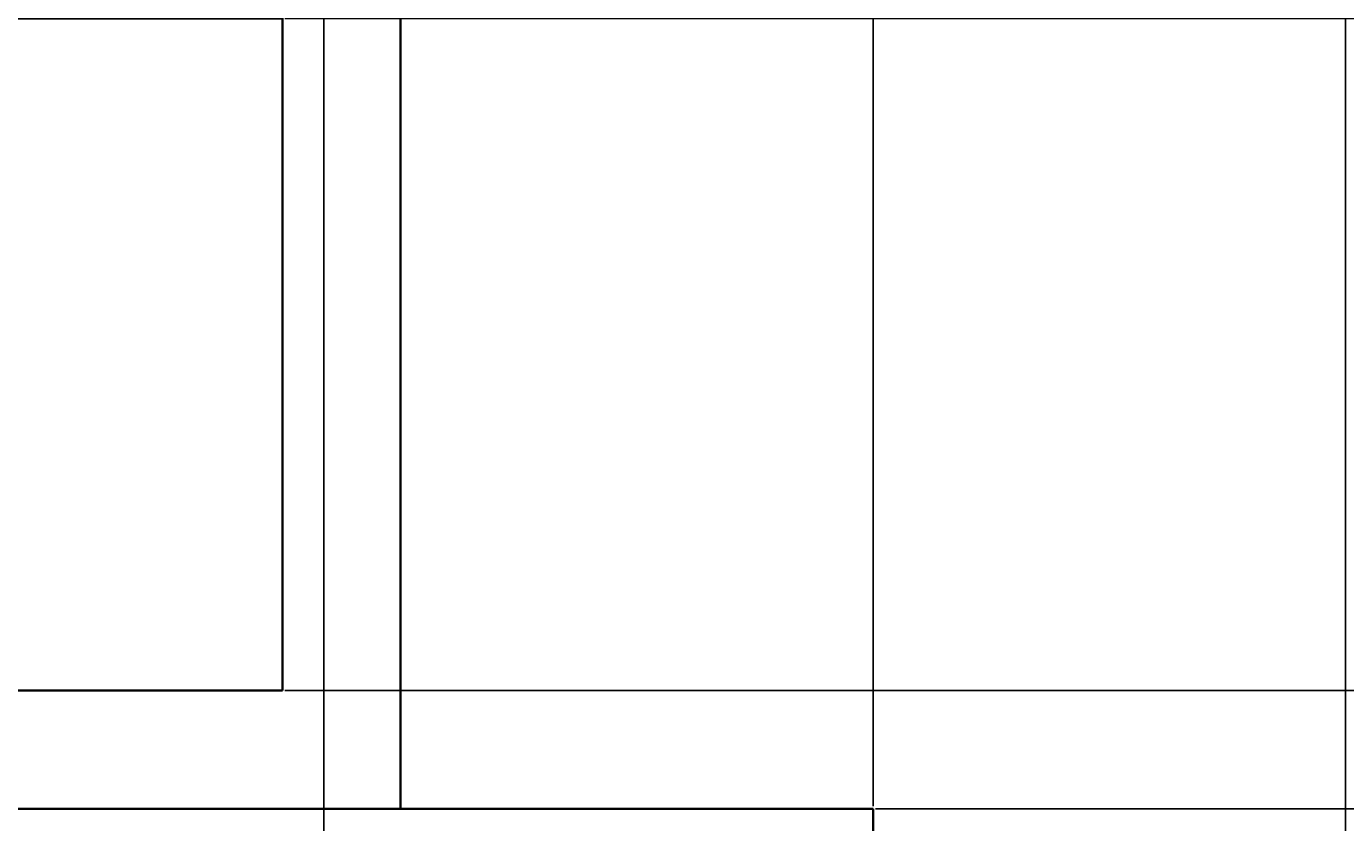
# Model space of a CAD drawing. Units: inches. Extents: x -6 to 289, y -8 to 323.
# Tile 65 of 107: x 238 to 271, y 139 to 159. Entities that reach past the tile are written whole.
import ezdxf

# ---------------------------------------------------------------- set-up
doc = ezdxf.new("R2010")
doc.units = ezdxf.units.IN
doc.header["$MEASUREMENT"] = 0
doc.layers.add('A-ANNO-DIMS', color=2, linetype='Continuous', lineweight=18)
doc.layers.add('A-ELEV', color=7, linetype='Continuous', lineweight=35)
doc.styles.get("Standard").update_dxf_attribs({"font": 'arial.ttf'})
doc.dimstyles.get("Standard").update_dxf_attribs({"dimtxt": 0.18, "dimasz": 0.18, "dimexe": 0.18, "dimexo": 0.0625, "dimgap": 0.09, "dimtad": 0, "dimtih": 1, "dimtoh": 1, "dimdec": 4, "dimzin": 0, "dimdsep": 46, "dimtxsty": 'Standard', "dimcen": 0.09, "dimadec": 0, "dimazin": 0, "dimtfac": 1, "dimtdec": 4, "dimtofl": 0, "dimtmove": 0, "dimatfit": 3, "dimfxl": 1, "dimtolj": 1, "dimtzin": 0, "dimarcsym": 0})

# ---------------------------------------------------------------- blocks, each defined once
blk = doc.blocks.new('*D15')
at = {"layer": 'A-ANNO-DIMS', "color": 0, "lineweight": -2, "transparency": 16777216}
for p, q in [((247.164, 162.411), (247.164, 322.969)), ((247.344, 322.789), (258.944, 322.789)), ((270.984, 322.789), (259.384, 322.789)), ((271.164, 7.351), (271.164, 322.969))]:
    blk.add_line(p, q, dxfattribs=at)
at = {"layer": 'A-ANNO-DIMS', "color": 0, "transparency": 16777216}
for points in [[(247.344, 322.819), (247.344, 322.759), (247.164, 322.789)], [(270.984, 322.819), (270.984, 322.759), (271.164, 322.789)]]:
    blk.add_solid(points, dxfattribs=at)
at = {"layer": 'Defpoints', "color": 0, "transparency": 16777216}
for p in [(271.164, 322.789), (247.164, 162.348), (271.164, 7.289)]:
    blk.add_point(p, dxfattribs=at)
at = {"layer": 'A-ANNO-DIMS', "color": 0, "transparency": 16777216, "insert": (259.164, 322.789), "char_height": 0.18, "attachment_point": 5}
blk.add_mtext('\\A1;24', dxfattribs=at)
blk = doc.blocks.new('*D24')
at = {"layer": 'A-ANNO-DIMS', "color": 0, "lineweight": -2, "transparency": 16777216}
for p, q in [((126.946, 178.654), (288.653, 178.654)), ((288.473, 178.474), (288.473, 159.153)), ((288.473, 139.469), (288.473, 158.789)), ((259.226, 139.289), (288.653, 139.289))]:
    blk.add_line(p, q, dxfattribs=at)
at = {"layer": 'A-ANNO-DIMS', "color": 0, "transparency": 16777216}
for points in [[(288.443, 178.474), (288.503, 178.474), (288.473, 178.654)], [(288.443, 139.469), (288.503, 139.469), (288.473, 139.289)]]:
    blk.add_solid(points, dxfattribs=at)
at = {"layer": 'Defpoints', "color": 0, "transparency": 16777216}
for p in [(126.883, 178.654), (288.473, 178.654), (259.164, 139.289)]:
    blk.add_point(p, dxfattribs=at)
at = {"layer": 'A-ANNO-DIMS', "color": 0, "transparency": 16777216, "insert": (288.473, 158.971), "char_height": 0.18, "attachment_point": 5}
blk.add_mtext('\\A1;39.365', dxfattribs=at)
blk = doc.blocks.new('*D81')
at = {"layer": 'A-ANNO-DIMS', "color": 0, "lineweight": -2, "transparency": 16777216}
for p, q in [((230.292, 68.842), (230.292, 322.969)), ((230.472, 322.789), (237.298, 322.789)), ((245.035, 322.789), (238.208, 322.789)), ((245.215, 66.286), (245.215, 322.969))]:
    blk.add_line(p, q, dxfattribs=at)
at = {"layer": 'A-ANNO-DIMS', "color": 0, "transparency": 16777216}
for points in [[(230.472, 322.819), (230.472, 322.759), (230.292, 322.789)], [(245.035, 322.819), (245.035, 322.759), (245.215, 322.789)]]:
    blk.add_solid(points, dxfattribs=at)
at = {"layer": 'Defpoints', "color": 0, "transparency": 16777216}
for p in [(245.215, 322.789), (230.292, 68.779), (245.215, 66.224)]:
    blk.add_point(p, dxfattribs=at)
at = {"layer": 'A-ANNO-DIMS', "color": 0, "transparency": 16777216, "insert": (237.753, 322.789), "char_height": 0.18, "attachment_point": 5}
blk.add_mtext('\\A1;14.923', dxfattribs=at)
blk = doc.blocks.new('*D82')
at = {"layer": 'A-ANNO-DIMS', "color": 0, "lineweight": -2, "transparency": 16777216}
for p, q in [((245.215, 66.286), (245.215, 322.969)), ((245.395, 322.789), (258.699, 322.789)), ((272.793, 322.789), (259.489, 322.789)), ((272.973, 66.286), (272.973, 322.969))]:
    blk.add_line(p, q, dxfattribs=at)
at = {"layer": 'A-ANNO-DIMS', "color": 0, "transparency": 16777216}
for points in [[(245.395, 322.819), (245.395, 322.759), (245.215, 322.789)], [(272.793, 322.819), (272.793, 322.759), (272.973, 322.789)]]:
    blk.add_solid(points, dxfattribs=at)
at = {"layer": 'Defpoints', "color": 0, "transparency": 16777216}
for p in [(272.973, 322.789), (245.215, 66.224), (272.973, 66.224)]:
    blk.add_point(p, dxfattribs=at)
at = {"layer": 'A-ANNO-DIMS', "color": 0, "transparency": 16777216, "insert": (259.094, 322.789), "char_height": 0.18, "attachment_point": 5}
blk.add_mtext('\\A1;27.76', dxfattribs=at)
blk = doc.blocks.new('*D100')
at = {"layer": 'A-ANNO-DIMS', "color": 0, "lineweight": -2, "transparency": 16777216}
for p, q in [((247.164, 162.411), (247.164, 322.969)), ((247.344, 322.789), (252.954, 322.789)), ((258.984, 322.789), (253.373, 322.789)), ((259.164, 139.351), (259.164, 322.969))]:
    blk.add_line(p, q, dxfattribs=at)
at = {"layer": 'A-ANNO-DIMS', "color": 0, "transparency": 16777216}
for points in [[(247.344, 322.819), (247.344, 322.759), (247.164, 322.789)], [(258.984, 322.819), (258.984, 322.759), (259.164, 322.789)]]:
    blk.add_solid(points, dxfattribs=at)
at = {"layer": 'Defpoints', "color": 0, "transparency": 16777216}
for p in [(259.164, 322.789), (247.164, 162.348), (259.164, 139.289)]:
    blk.add_point(p, dxfattribs=at)
at = {"layer": 'A-ANNO-DIMS', "color": 0, "transparency": 16777216, "insert": (253.164, 322.789), "char_height": 0.18, "attachment_point": 5}
blk.add_mtext('\\A1;12', dxfattribs=at)
blk = doc.blocks.new('*D101')
at = {"layer": 'A-ANNO-DIMS', "color": 0, "lineweight": -2, "transparency": 16777216}
for p, q in [((259.226, 139.289), (288.653, 139.289)), ((288.473, 139.109), (288.473, 133.469)), ((288.473, 127.469), (288.473, 133.108)), ((259.226, 127.289), (288.653, 127.289))]:
    blk.add_line(p, q, dxfattribs=at)
at = {"layer": 'A-ANNO-DIMS', "color": 0, "transparency": 16777216}
for points in [[(288.443, 139.109), (288.503, 139.109), (288.473, 139.289)], [(288.443, 127.469), (288.503, 127.469), (288.473, 127.289)]]:
    blk.add_solid(points, dxfattribs=at)
at = {"layer": 'Defpoints', "color": 0, "transparency": 16777216}
for p in [(259.164, 139.289), (288.473, 139.289), (259.164, 127.289)]:
    blk.add_point(p, dxfattribs=at)
at = {"layer": 'A-ANNO-DIMS', "color": 0, "transparency": 16777216, "insert": (288.473, 133.289), "char_height": 0.18, "attachment_point": 5}
blk.add_mtext('\\A1;12', dxfattribs=at)
blk = doc.blocks.new('*D102')
at = {"layer": 'A-ANNO-DIMS', "color": 0, "lineweight": -2, "transparency": 16777216}
for p, q in [((244.226, 142.289), (288.653, 142.289)), ((288.473, 142.109), (288.473, 140.971)), ((288.473, 139.469), (288.473, 140.607)), ((259.226, 139.289), (288.653, 139.289))]:
    blk.add_line(p, q, dxfattribs=at)
at = {"layer": 'A-ANNO-DIMS', "color": 0, "transparency": 16777216}
for points in [[(288.443, 142.109), (288.503, 142.109), (288.473, 142.289)], [(288.443, 139.469), (288.503, 139.469), (288.473, 139.289)]]:
    blk.add_solid(points, dxfattribs=at)
at = {"layer": 'Defpoints', "color": 0, "transparency": 16777216}
for p in [(244.164, 142.289), (288.473, 142.289), (259.164, 139.289)]:
    blk.add_point(p, dxfattribs=at)
at = {"layer": 'A-ANNO-DIMS', "color": 0, "transparency": 16777216, "insert": (288.473, 140.789), "char_height": 0.18, "attachment_point": 5}
blk.add_mtext('\\A1;3', dxfattribs=at)
blk = doc.blocks.new('*D103')
at = {"layer": 'A-ANNO-DIMS', "color": 0, "lineweight": -2, "transparency": 16777216}
for p, q in [((244.226, 159.348), (288.653, 159.348)), ((288.473, 159.168), (288.473, 151)), ((288.473, 142.469), (288.473, 150.637)), ((244.226, 142.289), (288.653, 142.289))]:
    blk.add_line(p, q, dxfattribs=at)
at = {"layer": 'A-ANNO-DIMS', "color": 0, "transparency": 16777216}
for points in [[(288.443, 159.168), (288.503, 159.168), (288.473, 159.348)], [(288.443, 142.469), (288.503, 142.469), (288.473, 142.289)]]:
    blk.add_solid(points, dxfattribs=at)
at = {"layer": 'Defpoints', "color": 0, "transparency": 16777216}
for p in [(244.164, 159.348), (288.473, 159.348), (244.164, 142.289)]:
    blk.add_point(p, dxfattribs=at)
at = {"layer": 'A-ANNO-DIMS', "color": 0, "transparency": 16777216, "insert": (288.473, 150.819), "char_height": 0.18, "attachment_point": 5}
blk.add_mtext('\\A1;17.06', dxfattribs=at)

msp = doc.modelspace()

# ---------------------------------------------------------------- linework, layer by layer
at = {"layer": 'A-ELEV'}
for p, q in [((247.1638, 139.2888), (247.1638, 247.2888)), ((115.1638, 139.2888), (259.1638, 139.2888)), ((259.1638, 127.2888), (259.1638, 139.2888))]:
    msp.add_line(p, q, dxfattribs=at)
for points in [[(247.1638, 139.2888), (115.1638, 139.2888), (115.1638, 162.3484), (247.1638, 162.3484)], [(244.1638, 142.2888), (118.1638, 142.2888), (118.1638, 159.3484), (244.1638, 159.3484)]]:
    msp.add_lwpolyline(points, close=True, dxfattribs=at)

# ---------------------------------------------------------------- dimensions: what is measured, and where the dimension line sits
at = {"layer": 'A-ANNO-DIMS'}
for base, p1, p2, override, picture, middle in [((245.2146, 322.7888), (230.2918, 68.7795), (245.2146, 66.2238), {"dimdec": 3, "dimlfac": 1, "dimrnd": 0, "dimzin": 0, "dimdsep": 46, "dimlunit": 2}, '*D81', (237.7532, 322.7888)), ((272.9733, 322.7888), (245.2146, 66.2238), (272.9733, 66.2238), {"dimdec": 2, "dimlfac": 1, "dimrnd": 0, "dimzin": 0, "dimdsep": 46, "dimlunit": 2}, '*D82', (259.0939, 322.7888)), ((271.1638, 322.7888), (247.1638, 162.3484), (271.1638, 7.2888), {"dimdec": 0, "dimlfac": 1, "dimrnd": 0, "dimzin": 0, "dimdsep": 46, "dimlunit": 2}, '*D15', (259.1638, 322.7888)), ((259.1638, 322.7888), (247.1638, 162.3484), (259.1638, 139.2888), {"dimdec": 0, "dimlfac": 1, "dimrnd": 0, "dimzin": 0, "dimdsep": 46, "dimlunit": 2}, '*D100', (253.1638, 322.7888))]:
    dim = msp.add_linear_dim(base=base, p1=p1, p2=p2, dimstyle='Standard', override=override, dxfattribs=at)
    dim.commit()
    dim.dimension.update_dxf_attribs({"geometry": picture, "text_midpoint": middle})
for base, p1, p2, override, picture, middle in [((288.4733, 178.654), (259.1638, 139.2888), (126.8835, 178.654), {"dimdec": 3, "dimlfac": 1, "dimrnd": 0, "dimzin": 0, "dimdsep": 46, "dimlunit": 2}, '*D24', (288.4733, 158.9714)), ((288.4733, 159.3484), (244.1638, 142.2888), (244.1638, 159.3484), {"dimdec": 2, "dimlfac": 1, "dimrnd": 0, "dimzin": 0, "dimdsep": 46, "dimlunit": 2}, '*D103', (288.4733, 150.8186)), ((288.4733, 142.2888), (259.1638, 139.2888), (244.1638, 142.2888), {"dimdec": 0, "dimlfac": 1, "dimrnd": 0, "dimzin": 0, "dimdsep": 46, "dimlunit": 2}, '*D102', (288.4733, 140.7888)), ((288.4733, 139.2888), (259.1638, 127.2888), (259.1638, 139.2888), {"dimdec": 0, "dimlfac": 1, "dimrnd": 0, "dimzin": 0, "dimdsep": 46, "dimlunit": 2}, '*D101', (288.4733, 133.2888))]:
    dim = msp.add_linear_dim(base=base, p1=p1, p2=p2, angle=90, dimstyle='Standard', override=override, dxfattribs=at)
    dim.commit()
    dim.dimension.update_dxf_attribs({"geometry": picture, "text_midpoint": middle})

doc.saveas('drawing.dxf')
